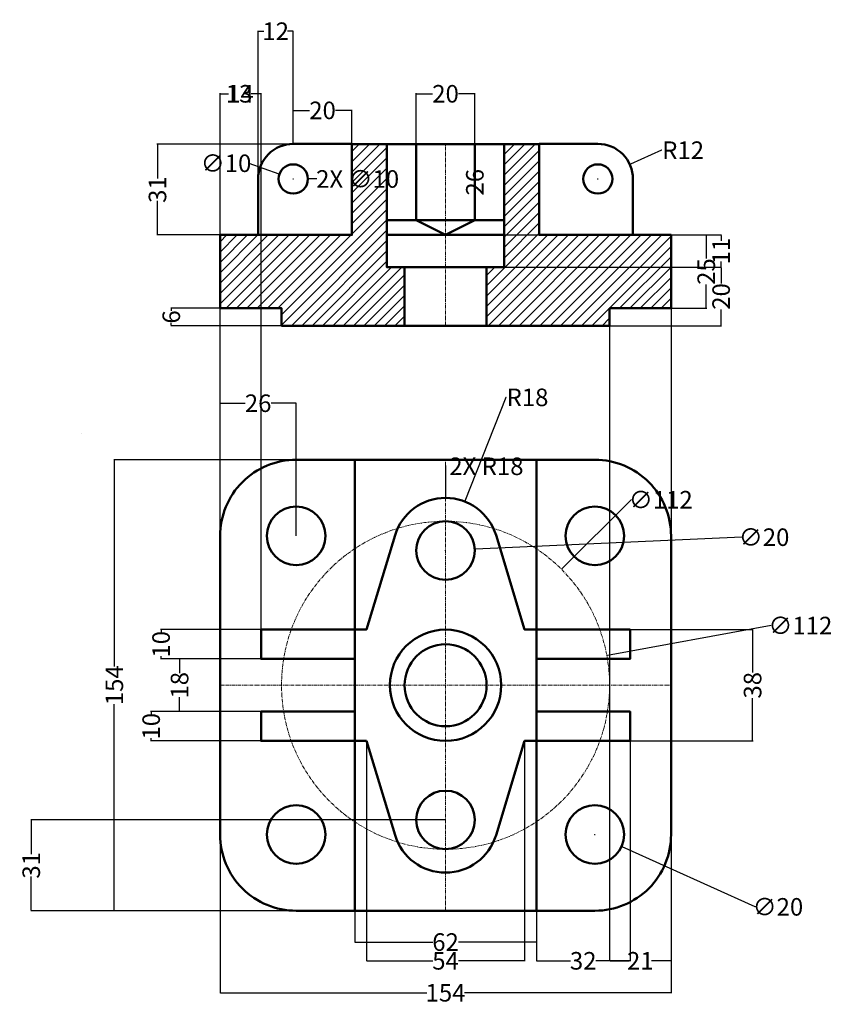
# Model space of a CAD drawing. Units: millimetres. Extents: x -8 to 269, y -225 to 111.
import ezdxf

# ---------------------------------------------------------------- set-up
doc = ezdxf.new("R2010")
doc.units = ezdxf.units.MM
doc.header["$MEASUREMENT"] = 0
doc.linetypes.add('CENTER', pattern=[2, 1.25, -0.25, 0.25, -0.25])
for name, color, linetype, lineweight in [('M-CNTR', 1, 'CENTER', 18), ('M-CONS', 9, 'Continuous', 13), ('M-DIMS', 2, 'Continuous', 25), ('M-HATC', 8, 'Continuous', 18), ('M-OUTL', 7, 'Continuous', 50)]:
    doc.layers.add(name, color=color, linetype=linetype, lineweight=lineweight)
doc.styles.get("Standard").update_dxf_attribs({"font": 'arial.ttf'})
doc.dimstyles.get("Standard").update_dxf_attribs({"dimtxt": 6, "dimasz": 0.18, "dimexe": 0.18, "dimexo": 0.0625, "dimgap": 0.09, "dimtad": 0, "dimtoh": 1, "dimdec": 0, "dimzin": 0, "dimdsep": 46, "dimtxsty": 'Standard', "dimcen": 0.09, "dimadec": 0, "dimazin": 0, "dimtfac": 1, "dimtdec": 0, "dimtofl": 0, "dimtmove": 0, "dimatfit": 3, "dimfxl": 1, "dimtolj": 1, "dimtzin": 0, "dimarcsym": 0})

# ---------------------------------------------------------------- blocks, each defined once
blk = doc.blocks.new('*D1')
at = {"layer": 'Defpoints', "color": 0, "lineweight": -2, "transparency": 16777216}
for p in [(147.26, 68.85), (147.26, 42.85), (147.26, 42.85)]:
    blk.add_point(p, dxfattribs=at)
at = {"layer": 'M-DIMS', "color": 0, "lineweight": -2, "transparency": 16777216}
for p, q in [((147.26, 68.67), (147.26, 60.28)), ((147.33, 68.85), (147.44, 68.85)), ((147.26, 43.03), (147.26, 51.41)), ((147.33, 42.85), (147.44, 42.85))]:
    blk.add_line(p, q, dxfattribs=at)
for points in [[(147.23, 68.67), (147.29, 68.67), (147.26, 68.85)], [(147.23, 43.03), (147.29, 43.03), (147.26, 42.85)]]:
    blk.add_solid(points, dxfattribs=at)
at = {"layer": 'M-DIMS', "color": 0, "transparency": 16777216, "insert": (147.26, 55.85), "char_height": 6, "attachment_point": 5, "rotation": 90}
blk.add_mtext('\\A1;26', dxfattribs=at)
blk = doc.blocks.new('*D2')
at = {"layer": 'Defpoints', "color": 0, "lineweight": -2, "transparency": 16777216}
for p in [(80.55, 58.64), (89.98, 55.3)]:
    blk.add_point(p, dxfattribs=at)
at = {"layer": 'M-DIMS', "color": 0, "lineweight": -2, "transparency": 16777216}
for p, q in [((69.95, 62.34), (70.13, 62.34)), ((70.13, 62.34), (80.38, 58.7)), ((85.17, 56.97), (85.35, 56.97)), ((85.26, 56.88), (85.26, 57.06))]:
    blk.add_line(p, q, dxfattribs=at)
blk.add_solid([(80.39, 58.73), (80.37, 58.67), (80.55, 58.64)], dxfattribs=at)
at = {"layer": 'M-DIMS', "color": 0, "transparency": 16777216, "insert": (62.31, 62.34), "char_height": 6, "attachment_point": 5}
blk.add_mtext('\\A1;∅10', dxfattribs=at)
blk = doc.blocks.new('*D3')
at = {"layer": 'Defpoints', "color": 0, "lineweight": -2, "transparency": 16777216}
for p in [(200.2, 61.92), (189.26, 56.97)]:
    blk.add_point(p, dxfattribs=at)
at = {"layer": 'M-DIMS', "color": 0, "lineweight": -2, "transparency": 16777216}
for p, q in [((210.97, 66.8), (200.36, 61.99)), ((211.15, 66.8), (210.97, 66.8)), ((189.17, 56.97), (189.35, 56.97)), ((189.26, 56.88), (189.26, 57.06))]:
    blk.add_line(p, q, dxfattribs=at)
blk.add_solid([(200.35, 62.02), (200.37, 61.97), (200.2, 61.92)], dxfattribs=at)
at = {"layer": 'M-DIMS', "color": 0, "transparency": 16777216, "insert": (218.38, 66.8), "char_height": 6, "attachment_point": 5}
blk.add_mtext('\\A1;R12', dxfattribs=at)
blk = doc.blocks.new('*D4')
at = {"layer": 'Defpoints', "color": 0, "lineweight": -2, "transparency": 16777216}
for p in [(85.26, 80.4), (85.26, 68.97), (105.26, 68.85)]:
    blk.add_point(p, dxfattribs=at)
at = {"layer": 'M-DIMS', "color": 0, "lineweight": -2, "transparency": 16777216}
for p, q in [((85.26, 69.03), (85.26, 80.58)), ((85.44, 80.4), (90.84, 80.4)), ((105.08, 80.4), (99.69, 80.4)), ((105.26, 68.91), (105.26, 80.58))]:
    blk.add_line(p, q, dxfattribs=at)
for points in [[(85.44, 80.43), (85.44, 80.37), (85.26, 80.4)], [(105.08, 80.43), (105.08, 80.37), (105.26, 80.4)]]:
    blk.add_solid(points, dxfattribs=at)
at = {"layer": 'M-DIMS', "color": 0, "transparency": 16777216, "insert": (95.26, 80.4), "char_height": 6, "attachment_point": 5}
blk.add_mtext('\\A1;20', dxfattribs=at)
blk = doc.blocks.new('*D5')
at = {"layer": 'Defpoints', "color": 0, "lineweight": -2, "transparency": 16777216}
for p in [(73.26, 107.44), (73.26, 68.97), (85.26, 68.97)]:
    blk.add_point(p, dxfattribs=at)
at = {"layer": 'M-DIMS', "color": 0, "lineweight": -2, "transparency": 16777216}
for p, q in [((73.26, 69.03), (73.26, 107.62)), ((85.26, 69.03), (85.26, 107.62)), ((73.44, 107.44), (75.19, 107.44)), ((85.08, 107.44), (83.34, 107.44))]:
    blk.add_line(p, q, dxfattribs=at)
for points in [[(73.44, 107.47), (73.44, 107.41), (73.26, 107.44)], [(85.08, 107.47), (85.08, 107.41), (85.26, 107.44)]]:
    blk.add_solid(points, dxfattribs=at)
at = {"layer": 'M-DIMS', "color": 0, "transparency": 16777216, "insert": (79.26, 107.44), "char_height": 6, "attachment_point": 5}
blk.add_mtext('\\A1;12', dxfattribs=at)
blk = doc.blocks.new('*D6')
at = {"layer": 'Defpoints', "color": 0, "lineweight": -2, "transparency": 16777216}
for p in [(81.26, 12.85), (43.6, 6.85), (81.26, 6.85)]:
    blk.add_point(p, dxfattribs=at)
at = {"layer": 'M-DIMS', "color": 0, "lineweight": -2, "transparency": 16777216}
for p, q in [((81.2, 12.85), (43.42, 12.85)), ((43.6, 12.67), (43.6, 11.92)), ((81.2, 6.85), (43.42, 6.85)), ((43.6, 7.03), (43.6, 7.78))]:
    blk.add_line(p, q, dxfattribs=at)
for points in [[(43.57, 12.67), (43.63, 12.67), (43.6, 12.85)], [(43.57, 7.03), (43.63, 7.03), (43.6, 6.85)]]:
    blk.add_solid(points, dxfattribs=at)
at = {"layer": 'M-DIMS', "color": 0, "transparency": 16777216, "insert": (43.6, 9.85), "char_height": 6, "attachment_point": 5, "rotation": 90}
blk.add_mtext('\\A1;6', dxfattribs=at)
blk = doc.blocks.new('*D7')
at = {"layer": 'Defpoints', "color": 0, "lineweight": -2, "transparency": 16777216}
for p in [(105.26, 68.85), (38.9, 37.85), (105.26, 37.85)]:
    blk.add_point(p, dxfattribs=at)
at = {"layer": 'M-DIMS', "color": 0, "lineweight": -2, "transparency": 16777216}
for p, q in [((105.2, 68.85), (38.72, 68.85)), ((38.9, 68.67), (38.9, 57.15)), ((38.9, 38.03), (38.9, 49.54)), ((105.2, 37.85), (38.72, 37.85))]:
    blk.add_line(p, q, dxfattribs=at)
for points in [[(38.87, 68.67), (38.93, 68.67), (38.9, 68.85)], [(38.87, 38.03), (38.93, 38.03), (38.9, 37.85)]]:
    blk.add_solid(points, dxfattribs=at)
at = {"layer": 'M-DIMS', "color": 0, "transparency": 16777216, "insert": (38.9, 53.35), "char_height": 6, "attachment_point": 5, "rotation": 90}
blk.add_mtext('\\A1;31', dxfattribs=at)
blk = doc.blocks.new('*D8')
at = {"layer": 'Defpoints', "color": 0, "lineweight": -2, "transparency": 16777216}
for p in [(214.26, 37.85), (214.26, 12.85), (226.27, 12.85)]:
    blk.add_point(p, dxfattribs=at)
at = {"layer": 'M-DIMS', "color": 0, "lineweight": -2, "transparency": 16777216}
for p, q in [((214.33, 37.85), (226.45, 37.85)), ((226.27, 37.67), (226.27, 29.81)), ((226.27, 13.03), (226.27, 20.89)), ((214.33, 12.85), (226.45, 12.85))]:
    blk.add_line(p, q, dxfattribs=at)
for points in [[(226.24, 37.67), (226.3, 37.67), (226.27, 37.85)], [(226.24, 13.03), (226.3, 13.03), (226.27, 12.85)]]:
    blk.add_solid(points, dxfattribs=at)
at = {"layer": 'M-DIMS', "color": 0, "transparency": 16777216, "insert": (226.27, 25.35), "char_height": 6, "attachment_point": 5, "rotation": 90}
blk.add_mtext('\\A1;25', dxfattribs=at)
blk = doc.blocks.new('*D9')
at = {"layer": 'Defpoints', "color": 0, "lineweight": -2, "transparency": 16777216}
for p in [(60.26, -19.62), (60.26, -64.94), (86.26, -64.94)]:
    blk.add_point(p, dxfattribs=at)
at = {"layer": 'M-DIMS', "color": 0, "lineweight": -2, "transparency": 16777216}
for p, q in [((60.26, -64.88), (60.26, -19.44)), ((60.44, -19.62), (68.83, -19.62)), ((86.08, -19.62), (77.7, -19.62)), ((86.26, -64.88), (86.26, -19.44))]:
    blk.add_line(p, q, dxfattribs=at)
for points in [[(60.44, -19.59), (60.44, -19.65), (60.26, -19.62)], [(86.08, -19.59), (86.08, -19.65), (86.26, -19.62)]]:
    blk.add_solid(points, dxfattribs=at)
at = {"layer": 'M-DIMS', "color": 0, "transparency": 16777216, "insert": (73.26, -19.62), "char_height": 6, "attachment_point": 5}
blk.add_mtext('\\A1;26', dxfattribs=at)
blk = doc.blocks.new('*D10')
at = {"layer": 'Defpoints', "color": 0, "lineweight": -2, "transparency": 16777216}
for p in [(143.84, -53.18), (137.26, -69.94)]:
    blk.add_point(p, dxfattribs=at)
at = {"layer": 'M-DIMS', "color": 0, "lineweight": -2, "transparency": 16777216}
for p, q in [((157.79, -17.61), (143.9, -53.02)), ((157.97, -17.61), (157.79, -17.61)), ((137.17, -69.94), (137.35, -69.94)), ((137.26, -70.03), (137.26, -69.85))]:
    blk.add_line(p, q, dxfattribs=at)
blk.add_solid([(143.88, -53), (143.93, -53.03), (143.84, -53.18)], dxfattribs=at)
at = {"layer": 'M-DIMS', "color": 0, "transparency": 16777216, "insert": (165.24, -17.61), "char_height": 6, "attachment_point": 5}
blk.add_mtext('\\A1;R18', dxfattribs=at)
blk = doc.blocks.new('*D11')
at = {"layer": 'Defpoints', "color": 0, "lineweight": -2, "transparency": 16777216}
for p in [(86.26, -38.94), (24.16, -192.94), (86.26, -192.94)]:
    blk.add_point(p, dxfattribs=at)
at = {"layer": 'M-DIMS', "color": 0, "lineweight": -2, "transparency": 16777216}
for p, q in [((86.2, -38.94), (23.98, -38.94)), ((24.16, -39.12), (24.16, -109.52)), ((24.16, -192.76), (24.16, -122.36)), ((86.2, -192.94), (23.98, -192.94))]:
    blk.add_line(p, q, dxfattribs=at)
for points in [[(24.13, -39.12), (24.19, -39.12), (24.16, -38.94)], [(24.13, -192.76), (24.19, -192.76), (24.16, -192.94)]]:
    blk.add_solid(points, dxfattribs=at)
at = {"layer": 'M-DIMS', "color": 0, "transparency": 16777216, "insert": (24.16, -115.94), "char_height": 6, "attachment_point": 5, "rotation": 90}
blk.add_mtext('\\A1;154', dxfattribs=at)
blk = doc.blocks.new('*D12')
at = {"layer": 'Defpoints', "color": 0, "lineweight": -2, "transparency": 16777216}
for p in [(60.26, -166.94), (214.26, -166.94), (214.26, -220.96)]:
    blk.add_point(p, dxfattribs=at)
at = {"layer": 'M-DIMS', "color": 0, "lineweight": -2, "transparency": 16777216}
for p, q in [((60.26, -167), (60.26, -221.14)), ((214.26, -167), (214.26, -221.14)), ((60.44, -220.96), (130.84, -220.96)), ((214.08, -220.96), (143.69, -220.96))]:
    blk.add_line(p, q, dxfattribs=at)
for points in [[(60.44, -220.93), (60.44, -220.99), (60.26, -220.96)], [(214.08, -220.93), (214.08, -220.99), (214.26, -220.96)]]:
    blk.add_solid(points, dxfattribs=at)
at = {"layer": 'M-DIMS', "color": 0, "transparency": 16777216, "insert": (137.26, -220.96), "char_height": 6, "attachment_point": 5}
blk.add_mtext('\\A1;154', dxfattribs=at)
blk = doc.blocks.new('*D13')
at = {"layer": 'Defpoints', "color": 0, "lineweight": -2, "transparency": 16777216}
for p in [(127.28, -70.39), (147.25, -69.49)]:
    blk.add_point(p, dxfattribs=at)
at = {"layer": 'M-DIMS', "color": 0, "lineweight": -2, "transparency": 16777216}
for p, q in [((238.39, -65.37), (147.43, -69.48)), ((137.17, -69.94), (137.35, -69.94)), ((137.26, -70.03), (137.26, -69.85))]:
    blk.add_line(p, q, dxfattribs=at)
blk.add_solid([(147.43, -69.45), (147.44, -69.51), (147.25, -69.49)], dxfattribs=at)
at = {"layer": 'M-DIMS', "color": 0, "transparency": 16777216, "insert": (246.03, -65.37), "char_height": 6, "attachment_point": 5}
blk.add_mtext('\\A1;∅20', dxfattribs=at)
blk = doc.blocks.new('*D14')
at = {"layer": 'Defpoints', "color": 0, "lineweight": -2, "transparency": 16777216}
for p in [(192.35, -105.84), (82.18, -126.04)]:
    blk.add_point(p, dxfattribs=at)
at = {"layer": 'M-DIMS', "color": 0, "lineweight": -2, "transparency": 16777216}
for p, q in [((248.46, -95.55), (192.52, -105.81)), ((137.17, -115.94), (137.35, -115.94)), ((137.26, -116.03), (137.26, -115.85))]:
    blk.add_line(p, q, dxfattribs=at)
blk.add_solid([(192.52, -105.78), (192.53, -105.84), (192.35, -105.84)], dxfattribs=at)
at = {"layer": 'M-DIMS', "color": 0, "transparency": 16777216, "insert": (258.42, -95.55), "char_height": 6, "attachment_point": 5}
blk.add_mtext('\\A1;∅112', dxfattribs=at)
blk = doc.blocks.new('*D15')
at = {"layer": 'Defpoints', "color": 0, "lineweight": -2, "transparency": 16777216}
for p in [(74.26, -96.94), (40.12, -106.94), (74.26, -106.94)]:
    blk.add_point(p, dxfattribs=at)
at = {"layer": 'M-DIMS', "color": 0, "lineweight": -2, "transparency": 16777216}
for p, q in [((74.2, -96.94), (39.94, -96.94)), ((40.12, -97.12), (40.12, -97.85)), ((74.2, -106.94), (39.94, -106.94)), ((40.12, -106.76), (40.12, -106.03))]:
    blk.add_line(p, q, dxfattribs=at)
for points in [[(40.09, -97.12), (40.15, -97.12), (40.12, -96.94)], [(40.09, -106.76), (40.15, -106.76), (40.12, -106.94)]]:
    blk.add_solid(points, dxfattribs=at)
at = {"layer": 'M-DIMS', "color": 0, "transparency": 16777216, "insert": (40.12, -101.94), "char_height": 6, "attachment_point": 5, "rotation": 90}
blk.add_mtext('\\A1;10', dxfattribs=at)
blk = doc.blocks.new('*D16')
at = {"layer": 'Defpoints', "color": 0, "lineweight": -2, "transparency": 16777216}
for p in [(106.26, -106.94), (46.44, -124.94), (106.26, -124.94)]:
    blk.add_point(p, dxfattribs=at)
at = {"layer": 'M-DIMS', "color": 0, "lineweight": -2, "transparency": 16777216}
for p, q in [((106.2, -106.94), (46.26, -106.94)), ((46.44, -107.12), (46.44, -111.83)), ((46.44, -124.76), (46.44, -120.05)), ((106.2, -124.94), (46.26, -124.94))]:
    blk.add_line(p, q, dxfattribs=at)
for points in [[(46.41, -107.12), (46.47, -107.12), (46.44, -106.94)], [(46.41, -124.76), (46.47, -124.76), (46.44, -124.94)]]:
    blk.add_solid(points, dxfattribs=at)
at = {"layer": 'M-DIMS', "color": 0, "transparency": 16777216, "insert": (46.44, -115.94), "char_height": 6, "attachment_point": 5, "rotation": 90}
blk.add_mtext('\\A1;18', dxfattribs=at)
blk = doc.blocks.new('*D17')
at = {"layer": 'Defpoints', "color": 0, "lineweight": -2, "transparency": 16777216}
for p in [(74.26, -124.94), (36.74, -134.94), (74.26, -134.94)]:
    blk.add_point(p, dxfattribs=at)
at = {"layer": 'M-DIMS', "color": 0, "lineweight": -2, "transparency": 16777216}
for p, q in [((74.2, -124.94), (36.56, -124.94)), ((36.74, -125.12), (36.74, -125.85)), ((36.74, -134.76), (36.74, -134.03)), ((74.2, -134.94), (36.56, -134.94))]:
    blk.add_line(p, q, dxfattribs=at)
for points in [[(36.71, -125.12), (36.77, -125.12), (36.74, -124.94)], [(36.71, -134.76), (36.77, -134.76), (36.74, -134.94)]]:
    blk.add_solid(points, dxfattribs=at)
at = {"layer": 'M-DIMS', "color": 0, "transparency": 16777216, "insert": (36.74, -129.94), "char_height": 6, "attachment_point": 5, "rotation": 90}
blk.add_mtext('\\A1;10', dxfattribs=at)
blk = doc.blocks.new('*D18')
at = {"layer": 'Defpoints', "color": 0, "lineweight": -2, "transparency": 16777216}
for p in [(106.26, -192.94), (168.26, -192.94), (168.26, -203.64)]:
    blk.add_point(p, dxfattribs=at)
at = {"layer": 'M-DIMS', "color": 0, "lineweight": -2, "transparency": 16777216}
for p, q in [((106.26, -193), (106.26, -203.82)), ((168.26, -193), (168.26, -203.82)), ((106.44, -203.64), (132.89, -203.64)), ((168.08, -203.64), (141.64, -203.64))]:
    blk.add_line(p, q, dxfattribs=at)
for points in [[(106.44, -203.61), (106.44, -203.67), (106.26, -203.64)], [(168.08, -203.61), (168.08, -203.67), (168.26, -203.64)]]:
    blk.add_solid(points, dxfattribs=at)
at = {"layer": 'M-DIMS', "color": 0, "transparency": 16777216, "insert": (137.26, -203.64), "char_height": 6, "attachment_point": 5}
blk.add_mtext('\\A1;62', dxfattribs=at)
blk = doc.blocks.new('*D19')
at = {"layer": 'Defpoints', "color": 0, "lineweight": -2, "transparency": 16777216}
for p in [(200.26, -96.94), (200.26, -134.94), (242.1, -134.94)]:
    blk.add_point(p, dxfattribs=at)
at = {"layer": 'M-DIMS', "color": 0, "lineweight": -2, "transparency": 16777216}
for p, q in [((200.33, -96.94), (242.28, -96.94)), ((242.1, -97.12), (242.1, -111.55)), ((242.1, -134.76), (242.1, -120.33)), ((200.33, -134.94), (242.28, -134.94))]:
    blk.add_line(p, q, dxfattribs=at)
for points in [[(242.07, -97.12), (242.13, -97.12), (242.1, -96.94)], [(242.07, -134.76), (242.13, -134.76), (242.1, -134.94)]]:
    blk.add_solid(points, dxfattribs=at)
at = {"layer": 'M-DIMS', "color": 0, "transparency": 16777216, "insert": (242.1, -115.94), "char_height": 6, "attachment_point": 5, "rotation": 90}
blk.add_mtext('\\A1;38', dxfattribs=at)
blk = doc.blocks.new('*D20')
at = {"layer": 'Defpoints', "color": 0, "lineweight": -2, "transparency": 16777216}
for p in [(179.15, -162.83), (197.38, -171.05)]:
    blk.add_point(p, dxfattribs=at)
at = {"layer": 'M-DIMS', "color": 0, "lineweight": -2, "transparency": 16777216}
for p, q in [((188.17, -166.94), (188.35, -166.94)), ((188.26, -167.03), (188.26, -166.85)), ((242.94, -191.62), (197.54, -171.13)), ((243.12, -191.62), (242.94, -191.62))]:
    blk.add_line(p, q, dxfattribs=at)
blk.add_solid([(197.56, -171.1), (197.53, -171.16), (197.38, -171.05)], dxfattribs=at)
at = {"layer": 'M-DIMS', "color": 0, "transparency": 16777216, "insert": (250.76, -191.62), "char_height": 6, "attachment_point": 5}
blk.add_mtext('\\A1;∅20', dxfattribs=at)
blk = doc.blocks.new('*D21')
at = {"layer": 'Defpoints', "color": 0, "lineweight": -2, "transparency": 16777216}
for p in [(-4.22, -161.94), (137.26, -161.94), (106.26, -192.94)]:
    blk.add_point(p, dxfattribs=at)
at = {"layer": 'M-DIMS', "color": 0, "lineweight": -2, "transparency": 16777216}
for p, q in [((137.2, -161.94), (-4.4, -161.94)), ((-4.22, -162.12), (-4.22, -173.63)), ((-4.22, -192.76), (-4.22, -181.25)), ((106.2, -192.94), (-4.4, -192.94))]:
    blk.add_line(p, q, dxfattribs=at)
for points in [[(-4.25, -162.12), (-4.19, -162.12), (-4.22, -161.94)], [(-4.25, -192.76), (-4.19, -192.76), (-4.22, -192.94)]]:
    blk.add_solid(points, dxfattribs=at)
at = {"layer": 'M-DIMS', "color": 0, "transparency": 16777216, "insert": (-4.22, -177.44), "char_height": 6, "attachment_point": 5, "rotation": 90}
blk.add_mtext('\\A1;31', dxfattribs=at)
blk = doc.blocks.new('*D22')
at = {"layer": 'Defpoints', "color": 0, "lineweight": -2, "transparency": 16777216}
for p in [(110.26, -134.94), (164.26, -134.94), (164.26, -210.04)]:
    blk.add_point(p, dxfattribs=at)
at = {"layer": 'M-DIMS', "color": 0, "lineweight": -2, "transparency": 16777216}
for p, q in [((110.26, -135), (110.26, -210.22)), ((164.26, -135), (164.26, -210.22)), ((110.44, -210.04), (132.89, -210.04)), ((164.08, -210.04), (141.64, -210.04))]:
    blk.add_line(p, q, dxfattribs=at)
for points in [[(110.44, -210.01), (110.44, -210.07), (110.26, -210.04)], [(164.08, -210.01), (164.08, -210.07), (164.26, -210.04)]]:
    blk.add_solid(points, dxfattribs=at)
at = {"layer": 'M-DIMS', "color": 0, "transparency": 16777216, "insert": (137.26, -210.04), "char_height": 6, "attachment_point": 5}
blk.add_mtext('\\A1;54', dxfattribs=at)
blk = doc.blocks.new('*D23')
at = {"layer": 'Defpoints', "color": 0, "lineweight": -2, "transparency": 16777216}
for p in [(74.26, 86.07), (60.26, -64.94), (74.26, -96.94)]:
    blk.add_point(p, dxfattribs=at)
at = {"layer": 'M-DIMS', "color": 0, "lineweight": -2, "transparency": 16777216}
for p, q in [((60.26, -64.88), (60.26, 86.25)), ((60.44, 86.07), (63.17, 86.07)), ((74.08, 86.07), (71.36, 86.07)), ((74.26, -96.88), (74.26, 86.25))]:
    blk.add_line(p, q, dxfattribs=at)
for points in [[(60.44, 86.1), (60.44, 86.04), (60.26, 86.07)], [(74.08, 86.1), (74.08, 86.04), (74.26, 86.07)]]:
    blk.add_solid(points, dxfattribs=at)
at = {"layer": 'M-DIMS', "color": 0, "transparency": 16777216, "insert": (67.26, 86.07), "char_height": 6, "attachment_point": 5}
blk.add_mtext('\\A1;14', dxfattribs=at)
blk = doc.blocks.new('*D24')
at = {"layer": 'Defpoints', "color": 0, "lineweight": -2, "transparency": 16777216}
for p in [(168.26, -124.94), (200.26, -124.94), (200.26, -210.04)]:
    blk.add_point(p, dxfattribs=at)
at = {"layer": 'M-DIMS', "color": 0, "lineweight": -2, "transparency": 16777216}
for p, q in [((168.26, -125), (168.26, -210.22)), ((200.26, -125), (200.26, -210.22)), ((168.44, -210.04), (179.91, -210.04)), ((200.08, -210.04), (188.62, -210.04))]:
    blk.add_line(p, q, dxfattribs=at)
for points in [[(168.44, -210.01), (168.44, -210.07), (168.26, -210.04)], [(200.08, -210.01), (200.08, -210.07), (200.26, -210.04)]]:
    blk.add_solid(points, dxfattribs=at)
at = {"layer": 'M-DIMS', "color": 0, "transparency": 16777216, "insert": (184.26, -210.04), "char_height": 6, "attachment_point": 5}
blk.add_mtext('\\A1;32', dxfattribs=at)
blk = doc.blocks.new('*D25')
at = {"layer": 'Defpoints', "color": 0, "lineweight": -2, "transparency": 16777216}
for p in [(214.26, 12.85), (193.26, 6.85), (214.26, -210.04)]:
    blk.add_point(p, dxfattribs=at)
at = {"layer": 'M-DIMS', "color": 0, "lineweight": -2, "transparency": 16777216}
for p, q in [((214.26, 12.79), (214.26, -210.22)), ((193.26, 6.79), (193.26, -210.22)), ((193.44, -210.04), (199.91, -210.04)), ((214.08, -210.04), (207.62, -210.04))]:
    blk.add_line(p, q, dxfattribs=at)
for points in [[(193.44, -210.01), (193.44, -210.07), (193.26, -210.04)], [(214.08, -210.01), (214.08, -210.07), (214.26, -210.04)]]:
    blk.add_solid(points, dxfattribs=at)
at = {"layer": 'M-DIMS', "color": 0, "transparency": 16777216, "insert": (203.76, -210.04), "char_height": 6, "attachment_point": 5}
blk.add_mtext('\\A1;21', dxfattribs=at)
blk = doc.blocks.new('*D26')
at = {"layer": 'Defpoints', "color": 0, "lineweight": -2, "transparency": 16777216}
for p in [(157.26, 37.85), (157.26, 26.85), (231.36, 26.85)]:
    blk.add_point(p, dxfattribs=at)
at = {"layer": 'M-DIMS', "color": 0, "lineweight": -2, "transparency": 16777216}
for p, q in [((157.33, 37.85), (231.54, 37.85)), ((231.36, 37.67), (231.36, 35.87)), ((231.36, 27.03), (231.36, 28.82)), ((157.33, 26.85), (231.54, 26.85))]:
    blk.add_line(p, q, dxfattribs=at)
for points in [[(231.33, 37.67), (231.39, 37.67), (231.36, 37.85)], [(231.33, 27.03), (231.39, 27.03), (231.36, 26.85)]]:
    blk.add_solid(points, dxfattribs=at)
at = {"layer": 'M-DIMS', "color": 0, "transparency": 16777216, "insert": (231.36, 32.35), "char_height": 6, "attachment_point": 5, "rotation": 90}
blk.add_mtext('\\A1;11', dxfattribs=at)
blk = doc.blocks.new('*D27')
at = {"layer": 'Defpoints', "color": 0, "lineweight": -2, "transparency": 16777216}
for p in [(151.26, 26.85), (151.26, 6.85), (231.36, 6.85)]:
    blk.add_point(p, dxfattribs=at)
at = {"layer": 'M-DIMS', "color": 0, "lineweight": -2, "transparency": 16777216}
for p, q in [((151.33, 26.85), (231.54, 26.85)), ((231.36, 26.67), (231.36, 21.28)), ((231.36, 7.03), (231.36, 12.42)), ((151.33, 6.85), (231.54, 6.85))]:
    blk.add_line(p, q, dxfattribs=at)
for points in [[(231.33, 26.67), (231.39, 26.67), (231.36, 26.85)], [(231.33, 7.03), (231.39, 7.03), (231.36, 6.85)]]:
    blk.add_solid(points, dxfattribs=at)
at = {"layer": 'M-DIMS', "color": 0, "transparency": 16777216, "insert": (231.36, 16.85), "char_height": 6, "attachment_point": 5, "rotation": 90}
blk.add_mtext('\\A1;20', dxfattribs=at)
blk = doc.blocks.new('*D28')
at = {"layer": 'Defpoints', "color": 0, "lineweight": -2, "transparency": 16777216}
for p in [(147.26, 86.07), (127.26, 68.97), (147.26, 68.97)]:
    blk.add_point(p, dxfattribs=at)
at = {"layer": 'M-DIMS', "color": 0, "lineweight": -2, "transparency": 16777216}
for p, q in [((127.26, 69.03), (127.26, 86.25)), ((127.44, 86.07), (132.84, 86.07)), ((147.08, 86.07), (141.69, 86.07)), ((147.26, 69.03), (147.26, 86.25))]:
    blk.add_line(p, q, dxfattribs=at)
for points in [[(127.44, 86.1), (127.44, 86.04), (127.26, 86.07)], [(147.08, 86.1), (147.08, 86.04), (147.26, 86.07)]]:
    blk.add_solid(points, dxfattribs=at)
at = {"layer": 'M-DIMS', "color": 0, "transparency": 16777216, "insert": (137.26, 86.07), "char_height": 6, "attachment_point": 5}
blk.add_mtext('\\A1;20', dxfattribs=at)
blk = doc.blocks.new('*D29')
at = {"layer": 'Defpoints', "color": 0, "lineweight": -2, "transparency": 16777216}
for p in [(73.26, 86.07), (60.26, 37.85), (73.26, 37.85)]:
    blk.add_point(p, dxfattribs=at)
at = {"layer": 'M-DIMS', "color": 0, "lineweight": -2, "transparency": 16777216}
for p, q in [((60.26, 37.91), (60.26, 86.25)), ((60.44, 86.07), (62.66, 86.07)), ((73.08, 86.07), (70.87, 86.07)), ((73.26, 37.91), (73.26, 86.25))]:
    blk.add_line(p, q, dxfattribs=at)
for points in [[(60.44, 86.1), (60.44, 86.04), (60.26, 86.07)], [(73.08, 86.1), (73.08, 86.04), (73.26, 86.07)]]:
    blk.add_solid(points, dxfattribs=at)
at = {"layer": 'M-DIMS', "color": 0, "transparency": 16777216, "insert": (66.76, 86.07), "char_height": 6, "attachment_point": 5}
blk.add_mtext('\\A1;13', dxfattribs=at)
blk = doc.blocks.new('*D30')
at = {"layer": 'Defpoints', "color": 0, "lineweight": -2, "transparency": 16777216}
for p in [(176.86, -76.34), (97.67, -155.54)]:
    blk.add_point(p, dxfattribs=at)
at = {"layer": 'M-DIMS', "color": 0, "lineweight": -2, "transparency": 16777216}
for p, q in [((200.62, -52.58), (176.99, -76.21)), ((200.8, -52.58), (200.62, -52.58)), ((137.17, -115.94), (137.35, -115.94)), ((137.26, -116.03), (137.26, -115.85))]:
    blk.add_line(p, q, dxfattribs=at)
blk.add_solid([(176.97, -76.19), (177.01, -76.24), (176.86, -76.34)], dxfattribs=at)
at = {"layer": 'M-DIMS', "color": 0, "transparency": 16777216, "insert": (210.75, -52.58), "char_height": 6, "attachment_point": 5}
blk.add_mtext('\\A1;∅112', dxfattribs=at)
blk = doc.blocks.new('*D31')
at = {"layer": 'Defpoints', "color": 0, "lineweight": -2, "transparency": 16777216}
for p in [(137.27, -51.94), (137.26, -69.94)]:
    blk.add_point(p, dxfattribs=at)
at = {"layer": 'M-DIMS', "color": 0, "lineweight": -2, "transparency": 16777216}
for p, q in [((137.45, -41.14), (137.27, -41.14)), ((137.27, -41.14), (137.27, -51.76)), ((137.17, -69.94), (137.35, -69.94)), ((137.26, -70.03), (137.26, -69.85))]:
    blk.add_line(p, q, dxfattribs=at)
blk.add_solid([(137.24, -51.76), (137.3, -51.76), (137.27, -51.94)], dxfattribs=at)
at = {"layer": 'M-DIMS', "color": 0, "transparency": 16777216, "insert": (151.21, -41.14), "char_height": 6, "attachment_point": 5}
blk.add_mtext('\\A1;2X R18', dxfattribs=at)
blk = doc.blocks.new('*D32')
at = {"layer": 'Defpoints', "color": 0, "lineweight": -2, "transparency": 16777216}
for p in [(80.26, 56.97), (90.26, 56.97)]:
    blk.add_point(p, dxfattribs=at)
at = {"layer": 'M-DIMS', "color": 0, "lineweight": -2, "transparency": 16777216}
for p, q in [((85.17, 56.97), (85.35, 56.97)), ((85.26, 56.88), (85.26, 57.06)), ((93.26, 56.97), (90.44, 56.97))]:
    blk.add_line(p, q, dxfattribs=at)
blk.add_solid([(90.44, 57), (90.44, 56.94), (90.26, 56.97)], dxfattribs=at)
at = {"layer": 'M-DIMS', "color": 0, "transparency": 16777216, "insert": (107.24, 56.97), "char_height": 6, "attachment_point": 5}
blk.add_mtext('\\A1;2X ∅10', dxfattribs=at)

msp = doc.modelspace()

# ---------------------------------------------------------------- hatches: boundary and pattern name
at = {"layer": 'M-HATC'}
h = msp.add_hatch(dxfattribs=at)
h.set_pattern_fill('ANSI31', color=256, scale=20)
h.paths.add_polyline_path([(123.26, 26.85), (117.26, 26.85), (117.26, 68.85), (105.26, 68.85), (105.26, 37.85), (60.26, 37.85), (60.26, 12.85), (81.26, 12.85), (81.26, 6.85), (123.26, 6.85)])
h.paths.add_polyline_path([(214.26, 37.85), (169.26, 37.85), (169.26, 68.85), (157.26, 68.85), (157.26, 26.85), (151.26, 26.85), (151.26, 6.85), (193.26, 6.85), (193.26, 12.85), (214.26, 12.85)])

# ---------------------------------------------------------------- linework, layer by layer
at = {"layer": 'M-CNTR'}
for p, q in [((123.26, 68.85), (123.26, 68.97)), ((137.26, 6.85), (137.26, 68.97)), ((151.26, 68.85), (151.26, 68.97)), ((137.26, -192.94), (137.26, -38.94)), ((60.26, -115.94), (214.26, -115.94))]:
    msp.add_line(p, q, dxfattribs=at)
msp.add_circle((137.26, -115.94), 56, dxfattribs=at)
at = {"layer": 'M-CONS'}
for p, q in [((12.88, -30.01), (12.88, -30.01)), ((86.26, -64.94), (86.26, -64.94)), ((200.26, -139.62), (200.26, -139.62))]:
    msp.add_line(p, q, dxfattribs=at)
at = {"layer": 'M-OUTL'}
for p, q in [((169.26, 68.85), (105.26, 68.85)), ((117.26, 42.85), (157.26, 42.85)), ((117.26, 37.85), (157.26, 37.85)), ((123.26, 6.85), (123.26, 26.85)), ((151.26, 6.85), (151.26, 26.85)), ((106.26, -192.94), (106.26, -38.94)), ((168.26, -192.94), (168.26, -38.94))]:
    msp.add_line(p, q, dxfattribs=at)
msp.add_lwpolyline([(201.26, 37.85), (201.26, 56.97, 0.414214), (189.26, 68.97), (169.26, 68.97), (169.26, 37.85), (214.26, 37.85), (214.26, 12.85), (193.26, 12.85), (193.26, 6.85), (81.26, 6.85), (81.26, 12.85), (60.26, 12.85), (60.26, 37.85), (105.26, 37.85), (105.26, 68.97), (85.26, 68.97, 0.414214), (73.26, 56.97), (73.26, 37.85)], format="xyb", dxfattribs=at)
for points in [[(157.26, 68.97), (157.26, 26.85), (117.26, 26.85), (117.26, 68.97)], [(147.26, 68.97), (147.26, 42.85), (137.26, 37.91), (127.26, 42.85), (127.26, 68.97)]]:
    msp.add_lwpolyline(points, dxfattribs=at)
for points in [[(60.26, -166.94, 0.414214), (86.26, -192.94), (188.26, -192.94, 0.414214), (214.26, -166.94), (214.26, -64.94, 0.414214), (188.26, -38.94), (86.26, -38.94, 0.414214), (60.26, -64.94)], [(110.26, -134.94), (74.26, -134.94), (74.26, -124.94), (86.41, -124.94), (106.26, -124.94), (106.26, -115.94), (106.26, -106.94), (86.41, -106.94), (74.26, -106.94), (74.26, -96.94), (110.25, -96.94), (120.04, -64.71, -0.741457), (154.49, -64.71), (164.26, -96.94), (200.26, -96.94), (200.26, -106.94), (168.26, -106.94), (168.26, -124.94), (200.26, -124.94), (200.26, -134.94), (164.26, -134.94), (154.49, -167.16, -0.741657), (120.04, -167.16)]]:
    msp.add_lwpolyline(points, format="xyb", close=True, dxfattribs=at)
for centre, radius in [((85.26, 56.97), 5), ((189.26, 56.97), 5), ((86.26, -64.94), 10), ((188.26, -64.94), 10), ((137.26, -69.94), 10), ((137.26, -115.94), 19), ((137.26, -115.94), 14), ((137.26, -161.94), 10), ((86.26, -166.94), 10), ((188.26, -166.94), 10)]:
    msp.add_circle(centre, radius, dxfattribs=at)

# ---------------------------------------------------------------- dimensions: what is measured, and where the dimension line sits
at = {"layer": 'M-DIMS'}
for base, p1, p2, override, picture, middle in [((73.26, 107.44), (85.26, 68.97), (73.26, 68.97), {"dimclrd": 0, "dimclre": 0, "dimclrt": 0}, '*D5', (79.26, 107.44)), ((74.26, 86.07), (60.26, -64.94), (74.26, -96.94), {"dimdec": 0, "dimlfac": 1, "dimrnd": 0, "dimzin": 0, "dimdsep": 46, "dimlunit": 2}, '*D23', (67.26, 86.07)), ((73.26, 86.07), (60.26, 37.85), (73.26, 37.85), {"dimdec": 0, "dimlfac": 1, "dimrnd": 0, "dimzin": 0, "dimdsep": 46, "dimlunit": 2}, '*D29', (66.76, 86.07)), ((147.26, 86.07), (127.26, 68.97), (147.26, 68.97), {"dimdec": 0, "dimlfac": 1, "dimrnd": 0, "dimzin": 0, "dimdsep": 46, "dimlunit": 2}, '*D28', (137.26, 86.07)), ((85.26, 80.4), (105.26, 68.85), (85.26, 68.97), {"dimclrd": 0, "dimclre": 0, "dimclrt": 0}, '*D4', (95.26, 80.4)), ((214.26, -210.04), (193.26, 6.85), (214.26, 12.85), {"dimdec": 0, "dimlfac": 1, "dimrnd": 0, "dimzin": 0, "dimdsep": 46, "dimlunit": 2}, '*D25', (203.76, -210.04)), ((60.26, -19.62), (86.26, -64.94), (60.26, -64.94), {"dimclrd": 0, "dimclre": 0, "dimclrt": 0}, '*D9', (73.26, -19.62)), ((200.26, -210.04), (168.26, -124.94), (200.26, -124.94), {"dimdec": 0, "dimlfac": 1, "dimrnd": 0, "dimzin": 0, "dimdsep": 46, "dimlunit": 2}, '*D24', (184.26, -210.04)), ((164.26, -210.04), (110.26, -134.94), (164.26, -134.94), {"dimdec": 0, "dimlfac": 1, "dimrnd": 0, "dimzin": 0, "dimdsep": 46, "dimlunit": 2}, '*D22', (137.26, -210.04)), ((214.26, -220.96), (60.26, -166.94), (214.26, -166.94), {"dimclrd": 0, "dimclre": 0, "dimclrt": 0}, '*D12', (137.26, -220.96)), ((168.26, -203.64), (106.26, -192.94), (168.26, -192.94), {"dimclrd": 0, "dimclre": 0, "dimclrt": 0}, '*D18', (137.26, -203.64))]:
    dim = msp.add_linear_dim(base=base, p1=p1, p2=p2, dimstyle='Standard', override=override, dxfattribs=at)
    dim.commit()
    dim.dimension.update_dxf_attribs({"geometry": picture, "text_midpoint": middle})
for center, mpoint, picture, middle in [((189.26, 56.97), (200.2, 61.92), '*D3', (218.38, 66.8)), ((137.26, -69.94), (143.84, -53.18), '*D10', (165.24, -17.61))]:
    dim = msp.add_radius_dim(center=center, mpoint=mpoint, dimstyle='Standard', override={"dimclrd": 0, "dimclre": 0, "dimclrt": 0}, dxfattribs=at)
    dim.commit()
    dim.dimension.update_dxf_attribs({"geometry": picture, "text_midpoint": middle, "dimtype": 164})
for base, p1, p2, override, picture, middle in [((38.9, 37.85), (105.26, 68.85), (105.26, 37.85), {"dimclrd": 0, "dimclre": 0, "dimclrt": 0}, '*D7', (38.9, 53.35)), ((147.26, 42.85), (147.26, 68.85), (147.26, 42.85), {"dimclrd": 0, "dimclre": 0, "dimclrt": 0}, '*D1', (147.26, 55.85)), ((231.36, 26.85), (157.26, 37.85), (157.26, 26.85), {"dimdec": 0, "dimlfac": 1, "dimrnd": 0, "dimzin": 0, "dimdsep": 46, "dimlunit": 2}, '*D26', (231.36, 32.35)), ((226.27, 12.85), (214.26, 37.85), (214.26, 12.85), {"dimclrd": 0, "dimclre": 0, "dimclrt": 0}, '*D8', (226.27, 25.35)), ((231.36, 6.85), (151.26, 26.85), (151.26, 6.85), {"dimdec": 0, "dimlfac": 1, "dimrnd": 0, "dimzin": 0, "dimdsep": 46, "dimlunit": 2}, '*D27', (231.36, 16.85)), ((43.6, 6.85), (81.26, 12.85), (81.26, 6.85), {"dimclrd": 0, "dimclre": 0, "dimclrt": 0}, '*D6', (43.6, 9.85)), ((24.16, -192.94), (86.26, -38.94), (86.26, -192.94), {"dimclrd": 0, "dimclre": 0, "dimclrt": 0}, '*D11', (24.16, -115.94)), ((40.12, -106.94), (74.26, -96.94), (74.26, -106.94), {"dimclrd": 0, "dimclre": 0, "dimclrt": 0}, '*D15', (40.12, -101.94)), ((242.1, -134.94), (200.26, -96.94), (200.26, -134.94), {"dimclrd": 0, "dimclre": 0, "dimclrt": 0}, '*D19', (242.1, -115.94)), ((46.44, -124.94), (106.26, -106.94), (106.26, -124.94), {"dimclrd": 0, "dimclre": 0, "dimclrt": 0}, '*D16', (46.44, -115.94)), ((36.74, -134.94), (74.26, -124.94), (74.26, -134.94), {"dimclrd": 0, "dimclre": 0, "dimclrt": 0}, '*D17', (36.74, -129.94)), ((-4.22, -161.94), (106.26, -192.94), (137.26, -161.94), {"dimdec": 0, "dimlfac": 1, "dimrnd": 0, "dimzin": 0, "dimdsep": 46, "dimlunit": 2}, '*D21', (-4.22, -177.44))]:
    dim = msp.add_linear_dim(base=base, p1=p1, p2=p2, angle=90, dimstyle='Standard', override=override, dxfattribs=at)
    dim.commit()
    dim.dimension.update_dxf_attribs({"geometry": picture, "text_midpoint": middle})
for p1, p2, override, picture, middle in [((89.98, 55.3), (80.55, 58.64), {"dimclrd": 0, "dimclre": 0, "dimclrt": 0}, '*D2', (62.31, 62.34)), ((97.67, -155.54), (176.86, -76.34), {"dimdec": 0, "dimlfac": 1, "dimrnd": 0, "dimzin": 0, "dimdsep": 46, "dimlunit": 2}, '*D30', (210.75, -52.58)), ((127.28, -70.39), (147.25, -69.49), {"dimclrd": 0, "dimclre": 0, "dimclrt": 0}, '*D13', (238.39, -65.37)), ((82.18, -126.04), (192.35, -105.84), {"dimclrd": 0, "dimclre": 0, "dimclrt": 0}, '*D14', (248.46, -95.55)), ((179.15, -162.83), (197.38, -171.05), {"dimclrd": 0, "dimclre": 0, "dimclrt": 0}, '*D20', (250.76, -191.62))]:
    dim = msp.add_diameter_dim_2p(p1=p1, p2=p2, dimstyle='Standard', override=override, dxfattribs=at)
    dim.commit()
    dim.dimension.update_dxf_attribs({"geometry": picture, "text_midpoint": middle, "dimtype": 163})
dim = msp.add_diameter_dim_2p(p1=(80.26, 56.97), p2=(90.26, 56.97), text='2X <>', dimstyle='Standard', override={"dimdec": 0, "dimlfac": 1, "dimrnd": 0, "dimzin": 0, "dimdsep": 46, "dimlunit": 2}, dxfattribs=at)
dim.commit()
dim.dimension.update_dxf_attribs({"geometry": '*D32', "text_midpoint": (93.26, 56.97), "dimtype": 163})
dim = msp.add_radius_dim(center=(137.26, -69.94), mpoint=(137.27, -51.94), text='2X <>', dimstyle='Standard', override={"dimdec": 0, "dimlfac": 1, "dimrnd": 0, "dimzin": 0, "dimdsep": 46, "dimlunit": 2}, dxfattribs=at)
dim.commit()
dim.dimension.update_dxf_attribs({"geometry": '*D31', "text_midpoint": (151.21, -41.14), "dimtype": 164})

doc.saveas('drawing.dxf')
